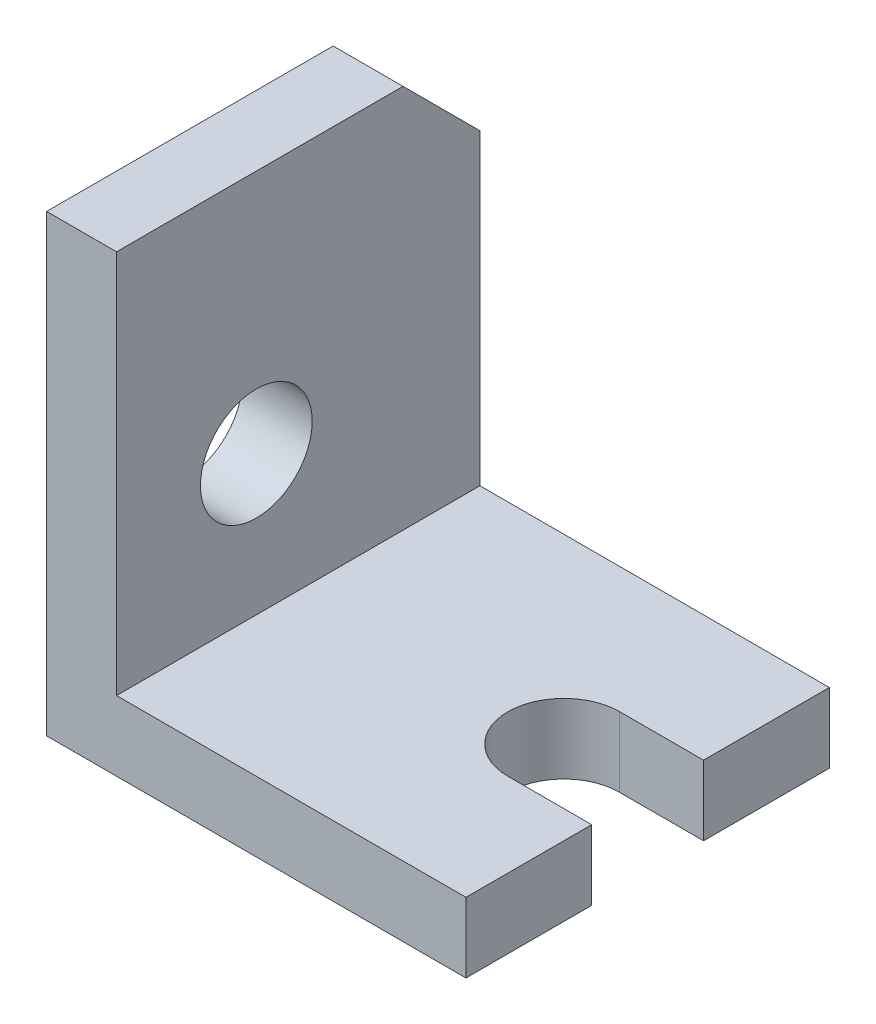
ISO-10303-21;
HEADER;
FILE_DESCRIPTION(('STEP AP214'),'2;1');
FILE_NAME('part.step','',(''),(''),'','','');
FILE_SCHEMA(('AUTOMOTIVE_DESIGN { 1 0 10303 214 1 1 1 1 }'));
ENDSEC;
DATA;
#1=APPLICATION_CONTEXT('core data for automotive mechanical design processes');
#2=APPLICATION_PROTOCOL_DEFINITION('international standard','automotive_design',2000,#1);
#3=PRODUCT_CONTEXT('',#1,'mechanical');
#4=PRODUCT('Part','Part','',(#3));
#5=PRODUCT_RELATED_PRODUCT_CATEGORY('part','',(#4));
#6=PRODUCT_DEFINITION_FORMATION('','',#4);
#7=PRODUCT_DEFINITION_CONTEXT('part definition',#1,'design');
#8=PRODUCT_DEFINITION('design','',#6,#7);
#9=PRODUCT_DEFINITION_SHAPE('','',#8);
#10=(LENGTH_UNIT() NAMED_UNIT(*) SI_UNIT(.MILLI.,.METRE.));
#11=(NAMED_UNIT(*) PLANE_ANGLE_UNIT() SI_UNIT($,.RADIAN.));
#12=(NAMED_UNIT(*) SI_UNIT($,.STERADIAN.) SOLID_ANGLE_UNIT());
#13=UNCERTAINTY_MEASURE_WITH_UNIT(LENGTH_MEASURE(1.E-05),#10,'distance_accuracy_value','');
#14=(GEOMETRIC_REPRESENTATION_CONTEXT(3) GLOBAL_UNCERTAINTY_ASSIGNED_CONTEXT((#13)) GLOBAL_UNIT_ASSIGNED_CONTEXT((#10,
#11,#12)) REPRESENTATION_CONTEXT('',''));
#15=CARTESIAN_POINT('',(0.,0.,0.));
#16=DIRECTION('',(0.,0.,1.));
#17=DIRECTION('',(1.,0.,0.));
#18=AXIS2_PLACEMENT_3D('',#15,#16,#17);
#19=CARTESIAN_POINT('',(60.,0.,26.));
#20=DIRECTION('',(0.,1.,0.));
#21=DIRECTION('',(0.,0.,1.));
#22=AXIS2_PLACEMENT_3D('',#19,#20,#21);
#23=PLANE('',#22);
#24=DIRECTION('',(1.,0.,0.));
#25=VECTOR('',#24,1.);
#26=CARTESIAN_POINT('',(48.,0.,-7.99999999999999));
#27=LINE('',#26,#25);
#28=CARTESIAN_POINT('',(48.,0.,-7.99999999999999));
#29=VERTEX_POINT('',#28);
#30=CARTESIAN_POINT('',(60.,0.,-7.99999999999999));
#31=VERTEX_POINT('',#30);
#32=EDGE_CURVE('E134',#29,#31,#27,.T.);
#33=ORIENTED_EDGE('',*,*,#32,.F.);
#34=CARTESIAN_POINT('',(48.,0.,0.));
#35=DIRECTION('',(0.,1.,0.));
#36=DIRECTION('',(0.,0.,1.));
#37=AXIS2_PLACEMENT_3D('',#34,#35,#36);
#38=CIRCLE('',#37,8.);
#39=CARTESIAN_POINT('',(48.,0.,8.));
#40=VERTEX_POINT('',#39);
#41=EDGE_CURVE('E126',#29,#40,#38,.T.);
#42=ORIENTED_EDGE('',*,*,#41,.T.);
#43=DIRECTION('',(1.,0.,0.));
#44=VECTOR('',#43,1.);
#45=CARTESIAN_POINT('',(48.,0.,8.));
#46=LINE('',#45,#44);
#47=CARTESIAN_POINT('',(60.,0.,8.));
#48=VERTEX_POINT('',#47);
#49=EDGE_CURVE('E138',#40,#48,#46,.T.);
#50=ORIENTED_EDGE('',*,*,#49,.T.);
#51=DIRECTION('',(0.,0.,-1.));
#52=VECTOR('',#51,1.);
#53=CARTESIAN_POINT('',(60.,0.,26.));
#54=LINE('',#53,#52);
#55=CARTESIAN_POINT('',(60.,0.,26.));
#56=VERTEX_POINT('',#55);
#57=EDGE_CURVE('E202',#56,#48,#54,.T.);
#58=ORIENTED_EDGE('',*,*,#57,.F.);
#59=DIRECTION('',(1.,0.,0.));
#60=VECTOR('',#59,1.);
#61=CARTESIAN_POINT('',(60.,0.,26.));
#62=LINE('',#61,#60);
#63=CARTESIAN_POINT('',(0.,0.,26.));
#64=VERTEX_POINT('',#63);
#65=EDGE_CURVE('E164',#64,#56,#62,.T.);
#66=ORIENTED_EDGE('',*,*,#65,.F.);
#67=DIRECTION('',(0.,0.,-1.));
#68=VECTOR('',#67,1.);
#69=CARTESIAN_POINT('',(0.,0.,26.));
#70=LINE('',#69,#68);
#71=CARTESIAN_POINT('',(0.,0.,-26.));
#72=VERTEX_POINT('',#71);
#73=EDGE_CURVE('E177',#64,#72,#70,.T.);
#74=ORIENTED_EDGE('',*,*,#73,.T.);
#75=DIRECTION('',(1.,0.,0.));
#76=VECTOR('',#75,1.);
#77=CARTESIAN_POINT('',(60.,0.,-26.));
#78=LINE('',#77,#76);
#79=CARTESIAN_POINT('',(60.,0.,-26.));
#80=VERTEX_POINT('',#79);
#81=EDGE_CURVE('E161',#72,#80,#78,.T.);
#82=ORIENTED_EDGE('',*,*,#81,.T.);
#83=EDGE_CURVE('E204',#31,#80,#54,.T.);
#84=ORIENTED_EDGE('',*,*,#83,.F.);
#85=EDGE_LOOP('',(#33,#42,#50,#58,#66,#74,#82,#84));
#86=FACE_BOUND('',#85,.T.);
#87=ADVANCED_FACE('F41',(#86),#23,.F.);
#88=CARTESIAN_POINT('',(60.,10.,26.));
#89=DIRECTION('',(-1.,0.,0.));
#90=DIRECTION('',(0.,-1.,0.));
#91=AXIS2_PLACEMENT_3D('',#88,#89,#90);
#92=PLANE('',#91);
#93=DIRECTION('',(0.,1.,0.));
#94=VECTOR('',#93,1.);
#95=CARTESIAN_POINT('',(60.,0.,-7.99999999999999));
#96=LINE('',#95,#94);
#97=CARTESIAN_POINT('',(60.,10.,-7.99999999999999));
#98=VERTEX_POINT('',#97);
#99=EDGE_CURVE('E165',#31,#98,#96,.T.);
#100=ORIENTED_EDGE('',*,*,#99,.F.);
#101=ORIENTED_EDGE('',*,*,#83,.T.);
#102=DIRECTION('',(0.,1.,0.));
#103=VECTOR('',#102,1.);
#104=CARTESIAN_POINT('',(60.,10.,-26.));
#105=LINE('',#104,#103);
#106=CARTESIAN_POINT('',(60.,10.,-26.));
#107=VERTEX_POINT('',#106);
#108=EDGE_CURVE('E185',#80,#107,#105,.T.);
#109=ORIENTED_EDGE('',*,*,#108,.T.);
#110=DIRECTION('',(0.,0.,-1.));
#111=VECTOR('',#110,1.);
#112=CARTESIAN_POINT('',(60.,10.,26.));
#113=LINE('',#112,#111);
#114=EDGE_CURVE('E199',#98,#107,#113,.T.);
#115=ORIENTED_EDGE('',*,*,#114,.F.);
#116=EDGE_LOOP('',(#100,#101,#109,#115));
#117=FACE_BOUND('',#116,.T.);
#118=ADVANCED_FACE('F236',(#117),#92,.F.);
#119=CARTESIAN_POINT('',(10.,10.,26.));
#120=DIRECTION('',(0.,-1.,0.));
#121=DIRECTION('',(0.,0.,-1.));
#122=AXIS2_PLACEMENT_3D('',#119,#120,#121);
#123=PLANE('',#122);
#124=DIRECTION('',(1.,0.,0.));
#125=VECTOR('',#124,1.);
#126=CARTESIAN_POINT('',(48.,10.,-7.99999999999999));
#127=LINE('',#126,#125);
#128=CARTESIAN_POINT('',(48.,10.,-7.99999999999999));
#129=VERTEX_POINT('',#128);
#130=EDGE_CURVE('E148',#129,#98,#127,.T.);
#131=ORIENTED_EDGE('',*,*,#130,.T.);
#132=ORIENTED_EDGE('',*,*,#114,.T.);
#133=DIRECTION('',(-1.,0.,0.));
#134=VECTOR('',#133,1.);
#135=CARTESIAN_POINT('',(10.,10.,-26.));
#136=LINE('',#135,#134);
#137=CARTESIAN_POINT('',(10.,10.,-26.));
#138=VERTEX_POINT('',#137);
#139=EDGE_CURVE('E183',#107,#138,#136,.T.);
#140=ORIENTED_EDGE('',*,*,#139,.T.);
#141=DIRECTION('',(0.,0.,-1.));
#142=VECTOR('',#141,1.);
#143=CARTESIAN_POINT('',(10.,10.,26.));
#144=LINE('',#143,#142);
#145=CARTESIAN_POINT('',(10.,10.,26.));
#146=VERTEX_POINT('',#145);
#147=EDGE_CURVE('E197',#146,#138,#144,.T.);
#148=ORIENTED_EDGE('',*,*,#147,.F.);
#149=DIRECTION('',(-1.,0.,0.));
#150=VECTOR('',#149,1.);
#151=CARTESIAN_POINT('',(10.,10.,26.));
#152=LINE('',#151,#150);
#153=CARTESIAN_POINT('',(60.,10.,26.));
#154=VERTEX_POINT('',#153);
#155=EDGE_CURVE('E171',#154,#146,#152,.T.);
#156=ORIENTED_EDGE('',*,*,#155,.F.);
#157=CARTESIAN_POINT('',(60.,10.,8.));
#158=VERTEX_POINT('',#157);
#159=EDGE_CURVE('E203',#154,#158,#113,.T.);
#160=ORIENTED_EDGE('',*,*,#159,.T.);
#161=DIRECTION('',(1.,0.,0.));
#162=VECTOR('',#161,1.);
#163=CARTESIAN_POINT('',(48.,10.,8.));
#164=LINE('',#163,#162);
#165=CARTESIAN_POINT('',(48.,10.,8.));
#166=VERTEX_POINT('',#165);
#167=EDGE_CURVE('E149',#166,#158,#164,.T.);
#168=ORIENTED_EDGE('',*,*,#167,.F.);
#169=CARTESIAN_POINT('',(48.,10.,0.));
#170=DIRECTION('',(0.,1.,0.));
#171=DIRECTION('',(0.,0.,1.));
#172=AXIS2_PLACEMENT_3D('',#169,#170,#171);
#173=CIRCLE('',#172,8.);
#174=EDGE_CURVE('E131',#129,#166,#173,.T.);
#175=ORIENTED_EDGE('',*,*,#174,.F.);
#176=EDGE_LOOP('',(#131,#132,#140,#148,#156,#160,#168,#175));
#177=FACE_BOUND('',#176,.T.);
#178=ADVANCED_FACE('F242',(#177),#123,.F.);
#179=ORIENTED_EDGE('',*,*,#57,.T.);
#180=DIRECTION('',(0.,1.,0.));
#181=VECTOR('',#180,1.);
#182=CARTESIAN_POINT('',(60.,0.,8.));
#183=LINE('',#182,#181);
#184=EDGE_CURVE('E133',#48,#158,#183,.T.);
#185=ORIENTED_EDGE('',*,*,#184,.T.);
#186=ORIENTED_EDGE('',*,*,#159,.F.);
#187=DIRECTION('',(0.,1.,0.));
#188=VECTOR('',#187,1.);
#189=CARTESIAN_POINT('',(60.,10.,26.));
#190=LINE('',#189,#188);
#191=EDGE_CURVE('E169',#56,#154,#190,.T.);
#192=ORIENTED_EDGE('',*,*,#191,.F.);
#193=EDGE_LOOP('',(#179,#185,#186,#192));
#194=FACE_BOUND('',#193,.T.);
#195=ADVANCED_FACE('F246',(#194),#92,.F.);
#196=CARTESIAN_POINT('',(9.99999999999999,65.,26.));
#197=DIRECTION('',(-1.,0.,0.));
#198=DIRECTION('',(0.,-1.,0.));
#199=AXIS2_PLACEMENT_3D('',#196,#197,#198);
#200=PLANE('',#199);
#201=CARTESIAN_POINT('',(10.,30.,6.));
#202=DIRECTION('',(1.,0.,0.));
#203=DIRECTION('',(0.,1.,0.));
#204=AXIS2_PLACEMENT_3D('',#201,#202,#203);
#205=CIRCLE('',#204,8.);
#206=CARTESIAN_POINT('',(10.,38.,6.));
#207=VERTEX_POINT('',#206);
#208=EDGE_CURVE('E155',#207,#207,#205,.T.);
#209=ORIENTED_EDGE('',*,*,#208,.F.);
#210=EDGE_LOOP('',(#209));
#211=FACE_BOUND('',#210,.T.);
#212=DIRECTION('',(0.,1.,0.));
#213=VECTOR('',#212,1.);
#214=CARTESIAN_POINT('',(9.99999999999999,65.,-26.));
#215=LINE('',#214,#213);
#216=CARTESIAN_POINT('',(10.,54.,-26.));
#217=VERTEX_POINT('',#216);
#218=EDGE_CURVE('E190',#138,#217,#215,.T.);
#219=ORIENTED_EDGE('',*,*,#218,.T.);
#220=DIRECTION('',(0.,0.707106781186549,0.707106781186546));
#221=VECTOR('',#220,1.);
#222=CARTESIAN_POINT('',(9.99999999999999,65.,-15.));
#223=LINE('',#222,#221);
#224=CARTESIAN_POINT('',(9.99999999999999,65.,-15.));
#225=VERTEX_POINT('',#224);
#226=EDGE_CURVE('E11',#217,#225,#223,.T.);
#227=ORIENTED_EDGE('',*,*,#226,.T.);
#228=DIRECTION('',(0.,0.,-1.));
#229=VECTOR('',#228,1.);
#230=CARTESIAN_POINT('',(9.99999999999999,65.,26.));
#231=LINE('',#230,#229);
#232=CARTESIAN_POINT('',(9.99999999999999,65.,26.));
#233=VERTEX_POINT('',#232);
#234=EDGE_CURVE('E192',#233,#225,#231,.T.);
#235=ORIENTED_EDGE('',*,*,#234,.F.);
#236=DIRECTION('',(0.,1.,0.));
#237=VECTOR('',#236,1.);
#238=CARTESIAN_POINT('',(9.99999999999999,65.,26.));
#239=LINE('',#238,#237);
#240=EDGE_CURVE('E172',#146,#233,#239,.T.);
#241=ORIENTED_EDGE('',*,*,#240,.F.);
#242=ORIENTED_EDGE('',*,*,#147,.T.);
#243=EDGE_LOOP('',(#219,#227,#235,#241,#242));
#244=FACE_BOUND('',#243,.T.);
#245=ADVANCED_FACE('F227',(#211,#244),#200,.F.);
#246=CARTESIAN_POINT('',(0.,65.,26.));
#247=DIRECTION('',(0.,-1.,0.));
#248=DIRECTION('',(0.,0.,-1.));
#249=AXIS2_PLACEMENT_3D('',#246,#247,#248);
#250=PLANE('',#249);
#251=ORIENTED_EDGE('',*,*,#234,.T.);
#252=DIRECTION('',(-1.,0.,0.));
#253=VECTOR('',#252,1.);
#254=CARTESIAN_POINT('',(0.,65.,-15.));
#255=LINE('',#254,#253);
#256=CARTESIAN_POINT('',(0.,65.,-15.));
#257=VERTEX_POINT('',#256);
#258=EDGE_CURVE('E210',#225,#257,#255,.T.);
#259=ORIENTED_EDGE('',*,*,#258,.T.);
#260=DIRECTION('',(0.,0.,-1.));
#261=VECTOR('',#260,1.);
#262=CARTESIAN_POINT('',(0.,65.,26.));
#263=LINE('',#262,#261);
#264=CARTESIAN_POINT('',(0.,65.,26.));
#265=VERTEX_POINT('',#264);
#266=EDGE_CURVE('E195',#265,#257,#263,.T.);
#267=ORIENTED_EDGE('',*,*,#266,.F.);
#268=DIRECTION('',(-1.,0.,0.));
#269=VECTOR('',#268,1.);
#270=CARTESIAN_POINT('',(0.,65.,26.));
#271=LINE('',#270,#269);
#272=EDGE_CURVE('E174',#233,#265,#271,.T.);
#273=ORIENTED_EDGE('',*,*,#272,.F.);
#274=EDGE_LOOP('',(#251,#259,#267,#273));
#275=FACE_BOUND('',#274,.T.);
#276=ADVANCED_FACE('F213',(#275),#250,.F.);
#277=CARTESIAN_POINT('',(0.,0.,26.));
#278=DIRECTION('',(1.,0.,0.));
#279=DIRECTION('',(0.,1.,0.));
#280=AXIS2_PLACEMENT_3D('',#277,#278,#279);
#281=PLANE('',#280);
#282=CARTESIAN_POINT('',(0.,30.,6.));
#283=DIRECTION('',(1.,0.,0.));
#284=DIRECTION('',(0.,1.,0.));
#285=AXIS2_PLACEMENT_3D('',#282,#283,#284);
#286=CIRCLE('',#285,8.);
#287=CARTESIAN_POINT('',(0.,38.,6.));
#288=VERTEX_POINT('',#287);
#289=EDGE_CURVE('E160',#288,#288,#286,.T.);
#290=ORIENTED_EDGE('',*,*,#289,.T.);
#291=EDGE_LOOP('',(#290));
#292=FACE_BOUND('',#291,.T.);
#293=ORIENTED_EDGE('',*,*,#266,.T.);
#294=DIRECTION('',(0.,-0.707106781186549,-0.707106781186546));
#295=VECTOR('',#294,1.);
#296=CARTESIAN_POINT('',(0.,65.,-15.));
#297=LINE('',#296,#295);
#298=CARTESIAN_POINT('',(0.,54.,-26.));
#299=VERTEX_POINT('',#298);
#300=EDGE_CURVE('E63',#257,#299,#297,.T.);
#301=ORIENTED_EDGE('',*,*,#300,.T.);
#302=DIRECTION('',(0.,-1.,0.));
#303=VECTOR('',#302,1.);
#304=CARTESIAN_POINT('',(0.,0.,-26.));
#305=LINE('',#304,#303);
#306=EDGE_CURVE('E166',#299,#72,#305,.T.);
#307=ORIENTED_EDGE('',*,*,#306,.T.);
#308=ORIENTED_EDGE('',*,*,#73,.F.);
#309=DIRECTION('',(0.,-1.,0.));
#310=VECTOR('',#309,1.);
#311=CARTESIAN_POINT('',(0.,0.,26.));
#312=LINE('',#311,#310);
#313=EDGE_CURVE('E180',#265,#64,#312,.T.);
#314=ORIENTED_EDGE('',*,*,#313,.F.);
#315=EDGE_LOOP('',(#293,#301,#307,#308,#314));
#316=FACE_BOUND('',#315,.T.);
#317=ADVANCED_FACE('F218',(#292,#316),#281,.F.);
#318=CARTESIAN_POINT('',(0.,0.,26.));
#319=DIRECTION('',(0.,0.,-1.));
#320=DIRECTION('',(-1.,0.,0.));
#321=AXIS2_PLACEMENT_3D('',#318,#319,#320);
#322=PLANE('',#321);
#323=ORIENTED_EDGE('',*,*,#65,.T.);
#324=ORIENTED_EDGE('',*,*,#191,.T.);
#325=ORIENTED_EDGE('',*,*,#155,.T.);
#326=ORIENTED_EDGE('',*,*,#240,.T.);
#327=ORIENTED_EDGE('',*,*,#272,.T.);
#328=ORIENTED_EDGE('',*,*,#313,.T.);
#329=EDGE_LOOP('',(#323,#324,#325,#326,#327,#328));
#330=FACE_BOUND('',#329,.T.);
#331=ADVANCED_FACE('F224',(#330),#322,.F.);
#332=CARTESIAN_POINT('',(0.,0.,-26.));
#333=DIRECTION('',(0.,0.,-1.));
#334=DIRECTION('',(-1.,0.,0.));
#335=AXIS2_PLACEMENT_3D('',#332,#333,#334);
#336=PLANE('',#335);
#337=ORIENTED_EDGE('',*,*,#306,.F.);
#338=DIRECTION('',(1.,0.,0.));
#339=VECTOR('',#338,1.);
#340=CARTESIAN_POINT('',(9.99999999999999,54.,-26.));
#341=LINE('',#340,#339);
#342=EDGE_CURVE('E49',#299,#217,#341,.T.);
#343=ORIENTED_EDGE('',*,*,#342,.T.);
#344=ORIENTED_EDGE('',*,*,#218,.F.);
#345=ORIENTED_EDGE('',*,*,#139,.F.);
#346=ORIENTED_EDGE('',*,*,#108,.F.);
#347=ORIENTED_EDGE('',*,*,#81,.F.);
#348=EDGE_LOOP('',(#337,#343,#344,#345,#346,#347));
#349=FACE_BOUND('',#348,.T.);
#350=ADVANCED_FACE('F261',(#349),#336,.T.);
#351=CARTESIAN_POINT('',(48.,0.,0.));
#352=DIRECTION('',(0.,1.,0.));
#353=DIRECTION('',(0.,0.,1.));
#354=AXIS2_PLACEMENT_3D('',#351,#352,#353);
#355=CYLINDRICAL_SURFACE('',#354,8.);
#356=ORIENTED_EDGE('',*,*,#174,.T.);
#357=DIRECTION('',(0.,1.,0.));
#358=VECTOR('',#357,1.);
#359=CARTESIAN_POINT('',(48.,0.,8.));
#360=LINE('',#359,#358);
#361=EDGE_CURVE('E122',#40,#166,#360,.T.);
#362=ORIENTED_EDGE('',*,*,#361,.F.);
#363=ORIENTED_EDGE('',*,*,#41,.F.);
#364=DIRECTION('',(0.,1.,0.));
#365=VECTOR('',#364,1.);
#366=CARTESIAN_POINT('',(48.,0.,-7.99999999999999));
#367=LINE('',#366,#365);
#368=EDGE_CURVE('E157',#29,#129,#367,.T.);
#369=ORIENTED_EDGE('',*,*,#368,.T.);
#370=EDGE_LOOP('',(#356,#362,#363,#369));
#371=FACE_BOUND('',#370,.T.);
#372=ADVANCED_FACE('F127',(#371),#355,.F.);
#373=CARTESIAN_POINT('',(48.,0.,-7.99999999999999));
#374=DIRECTION('',(0.,0.,1.));
#375=DIRECTION('',(1.,0.,0.));
#376=AXIS2_PLACEMENT_3D('',#373,#374,#375);
#377=PLANE('',#376);
#378=ORIENTED_EDGE('',*,*,#130,.F.);
#379=ORIENTED_EDGE('',*,*,#368,.F.);
#380=ORIENTED_EDGE('',*,*,#32,.T.);
#381=ORIENTED_EDGE('',*,*,#99,.T.);
#382=EDGE_LOOP('',(#378,#379,#380,#381));
#383=FACE_BOUND('',#382,.T.);
#384=ADVANCED_FACE('F266',(#383),#377,.T.);
#385=CARTESIAN_POINT('',(48.,0.,8.));
#386=DIRECTION('',(0.,0.,1.));
#387=DIRECTION('',(1.,0.,0.));
#388=AXIS2_PLACEMENT_3D('',#385,#386,#387);
#389=PLANE('',#388);
#390=ORIENTED_EDGE('',*,*,#167,.T.);
#391=ORIENTED_EDGE('',*,*,#184,.F.);
#392=ORIENTED_EDGE('',*,*,#49,.F.);
#393=ORIENTED_EDGE('',*,*,#361,.T.);
#394=EDGE_LOOP('',(#390,#391,#392,#393));
#395=FACE_BOUND('',#394,.T.);
#396=ADVANCED_FACE('F137',(#395),#389,.F.);
#397=CARTESIAN_POINT('',(0.,30.,6.));
#398=DIRECTION('',(1.,0.,0.));
#399=DIRECTION('',(0.,1.,0.));
#400=AXIS2_PLACEMENT_3D('',#397,#398,#399);
#401=CYLINDRICAL_SURFACE('',#400,8.);
#402=ORIENTED_EDGE('',*,*,#289,.F.);
#403=EDGE_LOOP('',(#402));
#404=FACE_BOUND('',#403,.T.);
#405=ORIENTED_EDGE('',*,*,#208,.T.);
#406=EDGE_LOOP('',(#405));
#407=FACE_BOUND('',#406,.T.);
#408=ADVANCED_FACE('F229',(#404,#407),#401,.F.);
#409=CARTESIAN_POINT('',(0.,65.,-15.));
#410=DIRECTION('',(0.,0.707106781186546,-0.707106781186549));
#411=DIRECTION('',(1.,0.,0.));
#412=AXIS2_PLACEMENT_3D('',#409,#410,#411);
#413=PLANE('',#412);
#414=ORIENTED_EDGE('',*,*,#226,.F.);
#415=ORIENTED_EDGE('',*,*,#342,.F.);
#416=ORIENTED_EDGE('',*,*,#300,.F.);
#417=ORIENTED_EDGE('',*,*,#258,.F.);
#418=EDGE_LOOP('',(#414,#415,#416,#417));
#419=FACE_BOUND('',#418,.T.);
#420=ADVANCED_FACE('F42',(#419),#413,.T.);
#421=CLOSED_SHELL('',(#87,#118,#178,#195,#245,#276,#317,#331,#350,#372,#384,#396,#408,#420));
#422=MANIFOLD_SOLID_BREP('B2',#421);
#423=ADVANCED_BREP_SHAPE_REPRESENTATION('',(#18,#422),#14);
#424=SHAPE_DEFINITION_REPRESENTATION(#9,#423);
ENDSEC;
END-ISO-10303-21;
